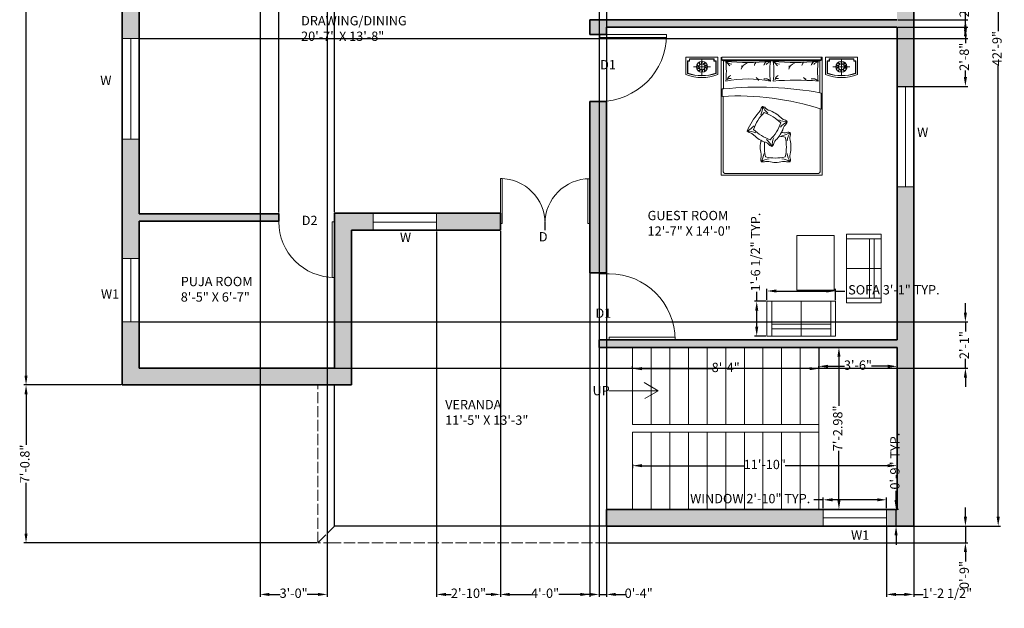
# Model space of a CAD drawing. Units: inches. Extents: x -34 to 523, y -544 to 92.
# Tile 1 of 2: x -11 to 518, y -544 to -227. Entities that reach past the tile are written whole.
import ezdxf

# ---------------------------------------------------------------- set-up
doc = ezdxf.new("R2010")
doc.units = ezdxf.units.IN
doc.linetypes.add('ACAD_ISO02W100', pattern=[15, 12, -3])
for name, color, linetype, lineweight in [('A-ANNO-DIMS', 2, 'Continuous', 18), ('A-ANNO-SYMB', 7, 'Continuous', 18), ('A-ANNO-TEXT', 7, 'Continuous', 18), ('A-AREA-IDEN', 7, 'Continuous', 25), ('A-DOOR', 4, 'Continuous', 18), ('A-FLOR', 7, 'Continuous', 25), ('A-FLOR-OVHD', 8, 'ACAD_ISO02W100', 18), ('A-FLOR-STRS', 7, 'Continuous', 18), ('A-GLAZ', 4, 'Continuous', 18), ('A-WALL', 7, 'Continuous', 35), ('furn', 28, 'Continuous', 18)]:
    doc.layers.add(name, color=color, linetype=linetype, lineweight=lineweight)
doc.layers.add('A-WALL-PATT', color=244, linetype='Continuous', lineweight=13, true_color=0x991b1e)
doc.styles.get("Standard").update_dxf_attribs({"font": 'arial.ttf'})
doc.dimstyles.new('ISO-25', dxfattribs={"dimtxt": 5, "dimasz": 5, "dimexe": 1.25, "dimexo": 0.625, "dimtad": 0, "dimlunit": 3, "dimtxsty": 'Standard', "dimcen": 2.5, "dimadec": 0, "dimazin": 0, "dimtfac": 1, "dimtmove": 0, "dimatfit": 3, "dimfxl": 1, "dimarcsym": 0})

# ---------------------------------------------------------------- blocks, each defined once
blk = doc.blocks.new('*U2')
for p, q in [((0, 0), (0, -6)), ((40, 0), (40, -6))]:
    blk.add_line(p, q)
blk.add_lwpolyline([(0, 0), (0, 40), (1.75, 40), (1.75, 0)], close=True)
blk.add_arc((0, 0), 40, 0, 90)
blk = doc.blocks.new('sofa-23')
at = {"color": 0, "linetype": 'ByBlock'}
for p, q in [((0, 0.74), (1.46, 0.74)), ((0, 0), (0, 0.74)), ((0.1, 0), (0.1, 0.74)), ((0.73, 0.74), (0.73, 0)), ((1.36, 0.74), (1.36, 0)), ((1.46, 0.74), (1.46, 0)), ((1.36, 0.25), (0.1, 0.25)), ((1.46, 0), (0, 0)), ((1.36, 0.15), (0.1, 0.15))]:
    blk.add_line(p, q, dxfattribs=at)
blk = doc.blocks.new('*D7')
at = {"layer": 'A-ANNO-DIMS', "color": 0, "lineweight": -2, "transparency": 16777216}
for p, q in [((418.12, -404.01), (418.12, -414.81)), ((460.12, -404.01), (460.12, -414.81)), ((423.12, -413.56), (431.86, -413.56)), ((455.12, -413.56), (446.39, -413.56))]:
    blk.add_line(p, q, dxfattribs=at)
at = {"layer": 'A-ANNO-DIMS', "color": 0, "transparency": 16777216}
for points in [[(423.12, -412.72), (423.12, -414.39), (418.12, -413.56)], [(455.12, -412.72), (455.12, -414.39), (460.12, -413.56)]]:
    blk.add_solid(points, dxfattribs=at)
at = {"layer": 'Defpoints', "color": 0, "transparency": 16777216}
for p in [(418.12, -403.38), (460.12, -403.38), (460.12, -413.56)]:
    blk.add_point(p, dxfattribs=at)
at = {"layer": 'A-ANNO-DIMS', "color": 0, "transparency": 16777216, "insert": (439.12, -413.56), "char_height": 5, "attachment_point": 5}
blk.add_mtext('3\'-6"', dxfattribs=at)
blk = doc.blocks.new('*D8')
at = {"layer": 'A-ANNO-DIMS', "color": 0, "lineweight": -2, "transparency": 16777216}
for p, q in [((318.12, -414.18), (318.12, -413.56)), ((323.12, -414.81), (360.85, -414.81)), ((413.12, -414.81), (375.4, -414.81)), ((418.12, -414.18), (418.12, -413.56))]:
    blk.add_line(p, q, dxfattribs=at)
at = {"layer": 'A-ANNO-DIMS', "color": 0, "transparency": 16777216}
for points in [[(323.12, -413.97), (323.12, -415.64), (318.12, -414.81)], [(413.12, -413.97), (413.12, -415.64), (418.12, -414.81)]]:
    blk.add_solid(points, dxfattribs=at)
at = {"layer": 'Defpoints', "color": 0, "transparency": 16777216}
for p in [(318.12, -414.81), (318.12, -414.81), (418.12, -414.81)]:
    blk.add_point(p, dxfattribs=at)
at = {"layer": 'A-ANNO-DIMS', "color": 0, "transparency": 16777216, "insert": (368.12, -414.81), "char_height": 5, "attachment_point": 5}
blk.add_mtext('8\'-4"', dxfattribs=at)
blk = doc.blocks.new('*D9')
at = {"layer": 'A-ANNO-DIMS', "color": 0, "lineweight": -2, "transparency": 16777216}
for p, q in [((418.75, -403.38), (430.17, -403.38)), ((428.92, -408.38), (428.92, -434.76)), ((428.92, -485.36), (428.92, -458.98)), ((418.75, -490.36), (430.17, -490.36))]:
    blk.add_line(p, q, dxfattribs=at)
at = {"layer": 'A-ANNO-DIMS', "color": 0, "transparency": 16777216}
for points in [[(428.09, -408.38), (429.75, -408.38), (428.92, -403.38)], [(428.09, -485.36), (429.75, -485.36), (428.92, -490.36)]]:
    blk.add_solid(points, dxfattribs=at)
at = {"layer": 'Defpoints', "color": 0, "transparency": 16777216}
for p in [(418.12, -403.38), (418.12, -490.36), (428.92, -490.36)]:
    blk.add_point(p, dxfattribs=at)
at = {"layer": 'A-ANNO-DIMS', "color": 0, "transparency": 16777216, "insert": (428.92, -446.87), "char_height": 5, "attachment_point": 5, "rotation": 90}
blk.add_mtext('7\'-2.98"', dxfattribs=at)
blk = doc.blocks.new('*D10')
at = {"layer": 'A-ANNO-DIMS', "color": 0, "lineweight": -2, "transparency": 16777216}
for p, q in [((318.12, -466.13), (318.12, -468.18)), ((323.12, -466.93), (378.2, -466.93)), ((455.12, -466.93), (400.04, -466.93)), ((460.12, -466.13), (460.12, -468.18))]:
    blk.add_line(p, q, dxfattribs=at)
at = {"layer": 'A-ANNO-DIMS', "color": 0, "transparency": 16777216}
for points in [[(323.12, -466.09), (323.12, -467.76), (318.12, -466.93)], [(455.12, -466.09), (455.12, -467.76), (460.12, -466.93)]]:
    blk.add_solid(points, dxfattribs=at)
at = {"layer": 'Defpoints', "color": 0, "transparency": 16777216}
for p in [(318.12, -465.51), (460.12, -465.51), (460.12, -466.93)]:
    blk.add_point(p, dxfattribs=at)
at = {"layer": 'A-ANNO-DIMS', "color": 0, "transparency": 16777216, "insert": (389.12, -466.93), "char_height": 5, "attachment_point": 5}
blk.add_mtext('11\'-10"', dxfattribs=at)
blk = doc.blocks.new('*D11')
at = {"layer": 'A-ANNO-DIMS', "color": 0, "lineweight": -2, "transparency": 16777216}
for p, q in [((43.5, -423.58), (-8.81, -423.58)), ((-7.56, -428.58), (-7.56, -455.82)), ((-7.56, -503.38), (-7.56, -476.14)), ((148.5, -508.38), (-8.81, -508.38))]:
    blk.add_line(p, q, dxfattribs=at)
at = {"layer": 'A-ANNO-DIMS', "color": 0, "transparency": 16777216}
for points in [[(-8.39, -428.58), (-6.73, -428.58), (-7.56, -423.58)], [(-8.39, -503.38), (-6.73, -503.38), (-7.56, -508.38)]]:
    blk.add_solid(points, dxfattribs=at)
at = {"layer": 'Defpoints', "color": 0, "transparency": 16777216}
for p in [(44.12, -423.58), (-7.56, -508.38), (149.12, -508.38)]:
    blk.add_point(p, dxfattribs=at)
at = {"layer": 'A-ANNO-DIMS', "color": 0, "transparency": 16777216, "insert": (-7.56, -465.98), "char_height": 5, "attachment_point": 5, "rotation": 90}
blk.add_mtext('7\'-0.8"', dxfattribs=at)
blk = doc.blocks.new('*D12')
at = {"layer": 'A-ANNO-DIMS', "color": 0, "lineweight": -2, "transparency": 16777216}
for p, q in [((0.5, 13.62), (-8.81, 13.62)), ((-7.56, 8.62), (-7.56, -192.86)), ((-7.56, -418.58), (-7.56, -217.1)), ((43.5, -423.58), (-8.81, -423.58))]:
    blk.add_line(p, q, dxfattribs=at)
at = {"layer": 'A-ANNO-DIMS', "color": 0, "transparency": 16777216}
for points in [[(-8.39, 8.62), (-6.73, 8.62), (-7.56, 13.62)], [(-8.39, -418.58), (-6.73, -418.58), (-7.56, -423.58)]]:
    blk.add_solid(points, dxfattribs=at)
at = {"layer": 'Defpoints', "color": 0, "transparency": 16777216}
for p in [(1.12, 13.62), (-7.56, -423.58), (44.12, -423.58)]:
    blk.add_point(p, dxfattribs=at)
at = {"layer": 'A-ANNO-DIMS', "color": 0, "transparency": 16777216, "insert": (-7.56, -204.98), "char_height": 5, "attachment_point": 5, "rotation": 90}
blk.add_mtext('36\'-5.2"', dxfattribs=at)
blk = doc.blocks.new('*D14')
at = {"layer": 'A-ANNO-DIMS', "color": 0, "lineweight": -2, "transparency": 16777216}
for p, q in [((469.75, 13.62), (515.68, 13.62)), ((514.43, 8.62), (514.43, -233.57)), ((514.43, -494.38), (514.43, -252.2)), ((469.75, -499.38), (515.68, -499.38))]:
    blk.add_line(p, q, dxfattribs=at)
at = {"layer": 'A-ANNO-DIMS', "color": 0, "transparency": 16777216}
for points in [[(513.6, 8.62), (515.26, 8.62), (514.43, 13.62)], [(513.6, -494.38), (515.26, -494.38), (514.43, -499.38)]]:
    blk.add_solid(points, dxfattribs=at)
at = {"layer": 'Defpoints', "color": 0, "transparency": 16777216}
for p in [(469.12, 13.62), (469.12, -499.38), (514.43, -499.38)]:
    blk.add_point(p, dxfattribs=at)
at = {"layer": 'A-ANNO-DIMS', "color": 0, "transparency": 16777216, "insert": (514.43, -242.88), "char_height": 5, "attachment_point": 5, "rotation": 90}
blk.add_mtext('42\'-9"', dxfattribs=at)
blk = doc.blocks.new('BED-DOUBLE')
for p, q in [((0.94, 61.53), (53.14, 61.53)), ((1.21, 61.99), (1.21, 46.38)), ((52.84, 61.99), (52.84, 44.35))]:
    blk.add_line(p, q)
for points in [[(0, 63.46), (0, 0), (54.08, 0), (54.08, 63.46)], [(53.58, 63.46), (53.58, 61.99), (0.31, 61.99), (0.31, 63.46), (54.08, 63.46)]]:
    blk.add_lwpolyline(points)
for points in [[(2.4, 50.65, 0.058596), (2.4, 61.1, 0.036889), (26.34, 61.1, 0.052163), (26.34, 50.65, 0.093111)], [(27.89, 50.65, 0.058596), (27.89, 61.1, 0.036648), (51.99, 61.1, 0.052163), (51.99, 50.65, 0.036967)], [(0.47, 46.38), (1.21, 46.38, -0.072944), (53.58, 44.2), (53.58, 35.53, 0.092568), (0.47, 42.4)]]:
    blk.add_lwpolyline(points, format="xyb", close=True)
for points in [[(0.94, 42.43), (0.94, 2.5, 0.414214), (2.5, 0.94), (51.58, 0.94, 0.414214), (53.14, 2.5), (53.14, 35.68)], [(21.24, 32.47, 0.091296), (22.19, 37.05, 0.091296), (25.07, 33.37, 0.091296)], [(17.36, 24.65, 0.111006), (26.29, 19.1, 0.119549), (31.92, 28.13, 0.107813), (23.02, 33.71)], [(22.97, 33.69, 0.121865), (17.36, 24.65, 0.121865)], [(18.5, 22.82, 0.091296), (13.92, 23.79, 0.091296), (17.61, 26.66, 0.091296)], [(27.19, 15.52, 0.159461), (28.4, 17.67, -0.076283), (29.36, 19, 0.115075), (33.28, 25.3, -0.076283), (34.06, 26.75, 0.159461), (35.45, 28.79)], [(30.88, 29.75, 0.091296), (35.45, 28.79, 0.091296), (31.76, 25.91, 0.091296)], [(32.56, 21.35, 0.091296), (36.96, 22.96, 0.091296), (35.34, 18.57, 0.091296)], [(36.96, 7.33, 0.159461), (36.85, 9.79, -0.076283), (36.96, 11.43, 0.115075), (36.96, 18.85, -0.076283), (36.85, 20.49, 0.159461), (36.96, 22.96)], [(23.79, 9.88, 0.111006), (34.31, 9.89, 0.119549), (34.31, 20.53, 0.033212), (31.08, 21.02)], [(28.14, 20.1, 0.091296), (27.19, 15.52, 0.091296), (24.3, 19.2)], [(25.72, 8.93, 0.091296), (21.33, 7.33, 0.091296), (22.94, 11.71, 0.091296)], [(35.34, 11.71, 0.091296), (36.96, 7.33, 0.091296), (32.56, 8.93)]]:
    blk.add_lwpolyline(points, format="xyb")
for centre, radius, start, end in [((0.94, 62.47), 0.938, 180, 270), ((7.95, 69.83), 10.35, 237.5379, 257.5233), ((-5.44, 51.33), 12.52, 36.4935, 51.2792), ((8.37, 58.13), 2.6, 335.8927, 16.1192), ((15.89, 54.9), 5.79, 96.6849, 148.3182), ((21.75, 58.2), 4.06, 141.8174, 169.8987), ((26.89, 57.62), 4.37, 130.5354, 160.3558), ((29.62, 53.94), 7.88, 114.6457, 134.1585), ((20.06, 51.33), 12.52, 36.4935, 51.2792), ((33.45, 69.83), 10.35, 237.5379, 257.5233), ((33.87, 58.13), 2.6, 335.8927, 16.1192), ((41.39, 54.9), 5.79, 96.6849, 148.3182), ((47.25, 58.2), 4.06, 141.8174, 169.8987), ((52.39, 57.62), 4.37, 130.5354, 160.3558), ((55.11, 53.94), 7.88, 114.6457, 134.1585), ((53.14, 62.47), 0.938, 270, 0), ((6.51, 50.41), 3.47, 114.2916, 160.9896), ((32.01, 50.41), 3.47, 114.2916, 160.9896), ((4.71, 49.68), 2.38, 76.4823, 128.5563), ((9.44, 43.38), 13.05, 36.2085, 45.0849), ((19.1, 51.09), 0.876, 353.7543, 77.2187), ((23.28, 47.66), 4.27, 44.406, 96.8342), ((24.08, 49.15), 2.71, 33.6349, 90.8456), ((30.2, 49.68), 2.38, 76.4823, 128.5563), ((34.94, 43.38), 13.05, 36.2085, 45.0849), ((44.59, 51.09), 0.876, 353.7543, 77.2187), ((48.78, 47.66), 4.27, 44.406, 96.8342), ((49.58, 49.15), 2.71, 33.6349, 90.8456), ((24.86, 34.13), 3.96, 132.4658, 168.7065), ((21.14, 33.37), 3.82, 37.2937, 74.0973), ((45.61, 10.83), 34.23, 138.3818, 157.7644), ((16.14, 37.37), 5.43, 315.5854, 333.0343), ((27.43, 40.04), 5.43, 233.2983, 250.7472), ((20.42, 19.44), 16.33, 45.1307, 71.3884), ((35.73, 34.9), 5.43, 225.7718, 243.2208), ((32.63, 26.46), 3.66, 39.4726, 79.6505), ((16.84, 26.47), 3.96, 222.6522, 258.8929), ((13.63, 17.74), 5.43, 45.7718, 63.2208), ((28.94, 33.2), 16.33, 225.1307, 251.3884), ((29.14, 7.07), 16.33, 77.0576, 78.7033), ((33.96, 28.3), 5.43, 257.6988, 275.1477), ((35.79, 19.49), 3.66, 71.3996, 111.5774), ((37.23, 15.14), 16.33, 166.8711, 193.1289), ((45.29, 15.25), 22.16, 173.1956, 194.0284), ((21.93, 12.6), 5.43, 53.2983, 70.7472), ((28.71, 19.79), 4.53, 218.7754, 250.3571), ((16.03, 10.26), 5.43, 355.0387, 12.4877), ((25.14, 8.39), 3.96, 159.3666, 195.6073), ((22.38, 11.14), 3.96, 254.5791, 290.8198), ((24.28, 2.04), 5.43, 77.6988, 95.1477), ((29.09, 23.26), 16.33, 257.0576, 283.3153), ((34.04, 2.07), 5.43, 85.2252, 102.6741), ((35.99, 11.75), 4.53, 250.7023, 282.284)]:
    blk.add_arc(centre, radius, start, end)
blk = doc.blocks.new('NIGHTSTAND-L')
for p, q in [((4.18, 5.76), (13.19, 5.76)), ((8.69, 1.26), (8.69, 10.27))]:
    blk.add_line(p, q)
blk.add_lwpolyline([(0, 1.56), (0, 10.94), (17.19, 10.94), (17.19, 1.56, -0.181818)], format="xyb", close=True)
for points in [[(1.97, 10), (1.97, 8.97), (0.94, 8.97)], [(2.06, 10), (2.06, 8.88), (0.94, 8.88)], [(1.97, 10), (15.22, 10)], [(1.97, 9.91), (15.22, 9.91)], [(15.13, 10), (15.13, 8.88), (16.26, 8.88)], [(15.22, 10), (15.22, 8.97), (16.26, 8.97)]]:
    blk.add_lwpolyline(points)
for points in [[(16.26, 8.97), (16.26, 2.22, -0.167087), (0.94, 2.22), (0.94, 8.97)], [(16.16, 8.97), (16.16, 2.28, -0.165559), (1.03, 2.28), (1.03, 8.97)]]:
    blk.add_lwpolyline(points, format="xyb")
for radius in [2.94, 1.6]:
    blk.add_circle((8.69, 5.76), radius)
for centre, radius, start, end in [((6.65, 6.51), 1.44, 232.3002, 292.538), ((7.6, 7.7), 1.89, 208.17, 254.4897), ((7.47, 7.56), 1.44, 196.3002, 256.538), ((8.95, 7.97), 1.89, 172.17, 218.4897), ((8.76, 7.93), 1.44, 160.3002, 220.538), ((10.19, 7.4), 1.89, 136.17, 182.4897), ((10.02, 7.47), 1.44, 124.3002, 184.538), ((10.86, 6.2), 1.89, 100.17, 146.4897), ((10.77, 6.36), 1.44, 88.3002, 148.538), ((10.7, 4.83), 1.89, 64.17, 110.4897), ((10.72, 5.02), 1.44, 52.3002, 112.538), ((9.9, 3.97), 1.44, 16.3002, 76.538), ((9.77, 3.83), 1.89, 28.17, 74.4897), ((6.67, 6.69), 1.89, 244.17, 290.4897), ((6.6, 5.17), 1.44, 268.3002, 328.538), ((6.51, 5.33), 1.89, 280.17, 326.4897), ((7.35, 4.06), 1.44, 304.3002, 4.538), ((7.18, 4.13), 1.89, 316.17, 2.4897), ((8.61, 3.6), 1.44, 340.3002, 40.538), ((8.42, 3.56), 1.89, 352.17, 38.4897)]:
    blk.add_arc(centre, radius, start, end)
blk = doc.blocks.new('NIGHTSTAND-R')
for p, q in [((13.02, 5.76), (4, 5.76)), ((8.51, 1.25), (8.51, 10.27))]:
    blk.add_line(p, q)
blk.add_lwpolyline([(17.19, 1.56), (17.19, 10.94), (0, 10.94), (0, 1.56, 0.181818)], format="xyb", close=True)
for points in [[(1.97, 10), (1.97, 8.97), (0.94, 8.97)], [(2.06, 10), (2.06, 8.88), (0.94, 8.88)], [(15.22, 10), (1.97, 10)], [(15.22, 9.91), (1.97, 9.91)], [(15.13, 10), (15.13, 8.88), (16.26, 8.88)], [(15.22, 10), (15.22, 8.97), (16.26, 8.97)]]:
    blk.add_lwpolyline(points)
for points in [[(0.94, 8.97), (0.94, 2.22, 0.167087), (16.26, 2.22), (16.26, 8.97)], [(1.03, 8.97), (1.03, 2.28, 0.165559), (16.16, 2.28), (16.16, 8.97)]]:
    blk.add_lwpolyline(points, format="xyb")
for radius in [2.94, 1.6]:
    blk.add_circle((8.51, 5.76), radius)
for centre, radius, start, end in [((6.47, 5.02), 1.44, 67.462, 127.6998), ((6.49, 4.83), 1.89, 69.5103, 115.83), ((7.42, 3.82), 1.89, 105.5103, 151.83), ((7.3, 3.96), 1.44, 103.462, 163.6998), ((6.43, 6.36), 1.44, 31.462, 91.6998), ((6.33, 6.19), 1.89, 33.5103, 79.83), ((7.17, 7.47), 1.44, 355.462, 55.6998), ((7, 7.39), 1.89, 357.5103, 43.83), ((8.43, 7.92), 1.44, 319.462, 19.6998), ((8.46, 8.05), 1.89, 321.5103, 7.83), ((10.76, 6.58), 1.44, 247.462, 307.6998), ((9.93, 7.64), 1.44, 283.462, 343.6998), ((9.81, 7.78), 1.89, 285.5103, 331.83), ((8.77, 3.55), 1.89, 141.5103, 187.83), ((8.58, 3.6), 1.44, 139.462, 199.6998), ((10.02, 4.13), 1.89, 177.5103, 223.83), ((9.84, 4.05), 1.44, 175.462, 235.6998), ((10.69, 5.33), 1.89, 213.5103, 259.83), ((10.59, 5.16), 1.44, 211.462, 271.6998), ((10.74, 6.77), 1.89, 249.5103, 295.83)]:
    blk.add_arc(centre, radius, start, end)
blk = doc.blocks.new('WIN-34IN')
blk.add_line((4.5, 34), (4.5, 0))
blk.add_lwpolyline([(9, 34), (9, 0), (0, 0), (0, 34)], close=True)
blk = doc.blocks.new('WIN-54IN')
blk.add_line((4.5, 54), (4.5, 0))
blk.add_lwpolyline([(0, 54), (9, 54), (9, 0), (0, 0)], close=True)
blk = doc.blocks.new('*D20')
at = {"layer": 'A-ANNO-DIMS', "color": 0, "lineweight": -2, "transparency": 16777216}
for p, q in [((420.49, -485.26), (415.49, -485.26)), ((420.49, -489.73), (420.49, -484.01)), ((449.49, -485.26), (425.49, -485.26)), ((454.49, -489.73), (454.49, -484.01))]:
    blk.add_line(p, q, dxfattribs=at)
at = {"layer": 'A-ANNO-DIMS', "color": 0, "transparency": 16777216}
for points in [[(425.49, -484.42), (425.49, -486.09), (420.49, -485.26)], [(449.49, -484.42), (449.49, -486.09), (454.49, -485.26)]]:
    blk.add_solid(points, dxfattribs=at)
at = {"layer": 'Defpoints', "color": 0, "transparency": 16777216}
for p in [(420.49, -485.26), (420.49, -490.36), (454.49, -490.36)]:
    blk.add_point(p, dxfattribs=at)
at = {"layer": 'A-ANNO-DIMS', "color": 0, "transparency": 16777216, "insert": (381.28, -485.26), "char_height": 5, "attachment_point": 5}
blk.add_mtext('WINDOW 2\'-10" TYP.', dxfattribs=at)
blk = doc.blocks.new('*D21')
at = {"layer": 'A-ANNO-DIMS', "color": 0, "lineweight": -2, "transparency": 16777216}
for p, q in [((459.59, -485.36), (459.59, -480.36)), ((455.11, -490.36), (460.84, -490.36)), ((459.59, -499.36), (459.59, -490.36)), ((455.11, -499.36), (460.84, -499.36)), ((459.59, -504.36), (459.59, -509.36))]:
    blk.add_line(p, q, dxfattribs=at)
at = {"layer": 'A-ANNO-DIMS', "color": 0, "transparency": 16777216}
for points in [[(458.75, -485.36), (460.42, -485.36), (459.59, -490.36)], [(458.75, -504.36), (460.42, -504.36), (459.59, -499.36)]]:
    blk.add_solid(points, dxfattribs=at)
at = {"layer": 'Defpoints', "color": 0, "transparency": 16777216}
for p in [(454.49, -490.36), (459.59, -490.36), (454.49, -499.36)]:
    blk.add_point(p, dxfattribs=at)
at = {"layer": 'A-ANNO-DIMS', "color": 0, "transparency": 16777216, "insert": (459.59, -464.49), "char_height": 5, "attachment_point": 5, "rotation": 90}
blk.add_mtext('0\'-9" TYP.', dxfattribs=at)
blk = doc.blocks.new('*D30')
at = {"layer": 'A-ANNO-DIMS', "color": 0, "lineweight": -2, "transparency": 16777216}
for p, q in [((390.29, -378.01), (390.29, -371.86)), ((395.29, -373.11), (422.1, -373.11)), ((427.1, -378.01), (427.1, -371.86)), ((427.1, -373.11), (432.1, -373.11))]:
    blk.add_line(p, q, dxfattribs=at)
at = {"layer": 'A-ANNO-DIMS', "color": 0, "transparency": 16777216}
for points in [[(395.29, -372.28), (395.29, -373.95), (390.29, -373.11)], [(422.1, -372.28), (422.1, -373.95), (427.1, -373.11)]]:
    blk.add_solid(points, dxfattribs=at)
at = {"layer": 'Defpoints', "color": 0, "transparency": 16777216}
for p in [(427.1, -373.11), (390.29, -378.64), (427.1, -378.64)]:
    blk.add_point(p, dxfattribs=at)
at = {"layer": 'A-ANNO-DIMS', "color": 0, "transparency": 16777216, "insert": (458.43, -373.11), "char_height": 5, "attachment_point": 5}
blk.add_mtext('SOFA 3\'-1" TYP.', dxfattribs=at)
blk = doc.blocks.new('*D31')
at = {"layer": 'A-ANNO-DIMS', "color": 0, "lineweight": -2, "transparency": 16777216}
for p, q in [((384.77, -378.64), (384.77, -373.64)), ((389.66, -378.64), (383.52, -378.64)), ((384.77, -392.29), (384.77, -383.64)), ((389.66, -397.29), (383.52, -397.29))]:
    blk.add_line(p, q, dxfattribs=at)
at = {"layer": 'A-ANNO-DIMS', "color": 0, "transparency": 16777216}
for points in [[(383.93, -383.64), (385.6, -383.64), (384.77, -378.64)], [(383.93, -392.29), (385.6, -392.29), (384.77, -397.29)]]:
    blk.add_solid(points, dxfattribs=at)
at = {"layer": 'Defpoints', "color": 0, "transparency": 16777216}
for p in [(384.77, -378.64), (390.29, -378.64), (390.29, -397.29)]:
    blk.add_point(p, dxfattribs=at)
at = {"layer": 'A-ANNO-DIMS', "color": 0, "transparency": 16777216, "insert": (384.77, -352.18), "char_height": 5, "attachment_point": 5, "rotation": 90}
blk.add_mtext('1\'-6 1/2" TYP.', dxfattribs=at)
blk = doc.blocks.new('*D32')
at = {"layer": 'A-ANNO-DIMS', "color": 0, "lineweight": -2, "transparency": 16777216}
for p, q in [((118.12, -168.01), (118.12, -537.33)), ((154.12, -168.01), (154.12, -537.33)), ((123.12, -536.08), (128.86, -536.08)), ((149.12, -536.08), (143.39, -536.08))]:
    blk.add_line(p, q, dxfattribs=at)
at = {"layer": 'A-ANNO-DIMS', "color": 0, "transparency": 16777216}
for points in [[(123.12, -535.25), (123.12, -536.92), (118.12, -536.08)], [(149.12, -535.25), (149.12, -536.92), (154.12, -536.08)]]:
    blk.add_solid(points, dxfattribs=at)
at = {"layer": 'Defpoints', "color": 0, "transparency": 16777216}
for p in [(118.12, -167.38), (154.12, -167.38), (154.12, -536.08)]:
    blk.add_point(p, dxfattribs=at)
at = {"layer": 'A-ANNO-DIMS', "color": 0, "transparency": 16777216, "insert": (136.12, -536.08), "char_height": 5, "attachment_point": 5}
blk.add_mtext('3\'-0"', dxfattribs=at)
blk = doc.blocks.new('*D33')
at = {"layer": 'A-ANNO-DIMS', "color": 0, "lineweight": -2, "transparency": 16777216}
for p, q in [((128.12, -330.95), (128.12, 42.7)), ((158.12, -330.76), (158.12, 42.7)), ((133.12, 41.45), (135.81, 41.45)), ((153.12, 41.45), (150.44, 41.45))]:
    blk.add_line(p, q, dxfattribs=at)
at = {"layer": 'A-ANNO-DIMS', "color": 0, "transparency": 16777216}
for points in [[(133.12, 42.29), (133.12, 40.62), (128.12, 41.45)], [(153.12, 42.29), (153.12, 40.62), (158.12, 41.45)]]:
    blk.add_solid(points, dxfattribs=at)
at = {"layer": 'Defpoints', "color": 0, "transparency": 16777216}
for p in [(158.12, 41.45), (128.12, -331.58), (158.12, -331.38)]:
    blk.add_point(p, dxfattribs=at)
at = {"layer": 'A-ANNO-DIMS', "color": 0, "transparency": 16777216, "insert": (143.12, 41.45), "char_height": 5, "attachment_point": 5}
blk.add_mtext('2\'-6"', dxfattribs=at)
blk = doc.blocks.new('*D34')
at = {"layer": 'A-ANNO-DIMS', "color": 0, "lineweight": -2, "transparency": 16777216}
for p, q in [((247.12, -341.01), (247.12, -537.33)), ((295.12, -341.08), (295.12, -537.33)), ((252.12, -536.08), (263.75, -536.08)), ((290.12, -536.08), (278.5, -536.08))]:
    blk.add_line(p, q, dxfattribs=at)
at = {"layer": 'A-ANNO-DIMS', "color": 0, "transparency": 16777216}
for points in [[(252.12, -535.25), (252.12, -536.92), (247.12, -536.08)], [(290.12, -535.25), (290.12, -536.92), (295.12, -536.08)]]:
    blk.add_solid(points, dxfattribs=at)
at = {"layer": 'Defpoints', "color": 0, "transparency": 16777216}
for p in [(247.12, -340.38), (295.12, -340.45), (295.12, -536.08)]:
    blk.add_point(p, dxfattribs=at)
at = {"layer": 'A-ANNO-DIMS', "color": 0, "transparency": 16777216, "insert": (271.12, -536.08), "char_height": 5, "attachment_point": 5}
blk.add_mtext('4\'-0"', dxfattribs=at)
blk = doc.blocks.new('*D37')
at = {"layer": 'A-ANNO-DIMS', "color": 0, "lineweight": -2, "transparency": 16777216}
for p, q in [((300.12, -168.01), (300.12, -537.33)), ((304.12, -164.01), (304.12, -537.33)), ((295.12, -536.08), (290.12, -536.08)), ((300.12, -536.08), (304.12, -536.08)), ((309.12, -536.08), (314.12, -536.08))]:
    blk.add_line(p, q, dxfattribs=at)
at = {"layer": 'A-ANNO-DIMS', "color": 0, "transparency": 16777216}
for points in [[(295.12, -535.25), (295.12, -536.92), (300.12, -536.08)], [(309.12, -535.25), (309.12, -536.92), (304.12, -536.08)]]:
    blk.add_solid(points, dxfattribs=at)
at = {"layer": 'Defpoints', "color": 0, "transparency": 16777216}
for p in [(304.12, -163.38), (300.12, -167.38), (304.12, -536.08)]:
    blk.add_point(p, dxfattribs=at)
at = {"layer": 'A-ANNO-DIMS', "color": 0, "transparency": 16777216, "insert": (321.4, -536.08), "char_height": 5, "attachment_point": 5}
blk.add_mtext('0\'-4"', dxfattribs=at)
blk = doc.blocks.new('*D41')
at = {"layer": 'A-ANNO-DIMS', "color": 0, "lineweight": -2, "transparency": 16777216}
for p, q in [((53.75, -167.38), (498.07, -167.38)), ((496.82, -172.38), (496.82, -193.25)), ((496.82, -232.53), (496.82, -211.67)), ((53.78, -237.53), (498.07, -237.53))]:
    blk.add_line(p, q, dxfattribs=at)
at = {"layer": 'A-ANNO-DIMS', "color": 0, "transparency": 16777216}
for points in [[(495.99, -172.38), (497.66, -172.38), (496.82, -167.38)], [(495.99, -232.53), (497.66, -232.53), (496.82, -237.53)]]:
    blk.add_solid(points, dxfattribs=at)
at = {"layer": 'Defpoints', "color": 0, "transparency": 16777216}
for p in [(53.12, -167.38), (53.16, -237.53), (496.82, -237.53)]:
    blk.add_point(p, dxfattribs=at)
at = {"layer": 'A-ANNO-DIMS', "color": 0, "transparency": 16777216, "insert": (496.82, -202.46), "char_height": 5, "attachment_point": 5, "rotation": 90}
blk.add_mtext('5\'-10"', dxfattribs=at)
blk = doc.blocks.new('*D42')
at = {"layer": 'A-ANNO-DIMS', "color": 0, "lineweight": -2, "transparency": 16777216}
for p, q in [((496.82, -384.72), (496.82, -379.72)), ((53.75, -389.72), (498.07, -389.72)), ((496.82, -389.72), (496.82, -394.84)), ((496.82, -414.58), (496.82, -409.46)), ((53.75, -414.58), (498.07, -414.58)), ((496.82, -419.58), (496.82, -424.58))]:
    blk.add_line(p, q, dxfattribs=at)
at = {"layer": 'A-ANNO-DIMS', "color": 0, "transparency": 16777216}
for points in [[(495.99, -384.72), (497.66, -384.72), (496.82, -389.72)], [(495.99, -419.58), (497.66, -419.58), (496.82, -414.58)]]:
    blk.add_solid(points, dxfattribs=at)
at = {"layer": 'Defpoints', "color": 0, "transparency": 16777216}
for p in [(53.12, -389.72), (53.12, -414.58), (496.82, -414.58)]:
    blk.add_point(p, dxfattribs=at)
at = {"layer": 'A-ANNO-DIMS', "color": 0, "transparency": 16777216, "insert": (496.82, -402.15), "char_height": 5, "attachment_point": 5, "rotation": 90}
blk.add_mtext('2\'-1"', dxfattribs=at)
blk = doc.blocks.new('*D44')
at = {"layer": 'A-ANNO-DIMS', "color": 0, "lineweight": -2, "transparency": 16777216}
for p, q in [((460.75, -231.38), (498.07, -231.38)), ((496.82, -236.38), (496.82, -239.98)), ((496.82, -258.2), (496.82, -254.61)), ((460.75, -263.2), (498.07, -263.2))]:
    blk.add_line(p, q, dxfattribs=at)
at = {"layer": 'A-ANNO-DIMS', "color": 0, "transparency": 16777216}
for points in [[(495.99, -236.38), (497.66, -236.38), (496.82, -231.38)], [(495.99, -258.2), (497.66, -258.2), (496.82, -263.2)]]:
    blk.add_solid(points, dxfattribs=at)
at = {"layer": 'Defpoints', "color": 0, "transparency": 16777216}
for p in [(460.12, -231.38), (460.12, -263.2), (496.82, -263.2)]:
    blk.add_point(p, dxfattribs=at)
at = {"layer": 'A-ANNO-DIMS', "color": 0, "transparency": 16777216, "insert": (496.82, -247.29), "char_height": 5, "attachment_point": 5, "rotation": 90}
blk.add_mtext('2\'-8"', dxfattribs=at)
blk = doc.blocks.new('*D45')
at = {"layer": 'A-ANNO-DIMS', "color": 0, "lineweight": -2, "transparency": 16777216}
for p, q in [((212.88, -341.18), (212.88, -537.33)), ((247.12, -341.01), (247.12, -537.33)), ((217.88, -536.08), (220.75, -536.08)), ((242.12, -536.08), (239.26, -536.08))]:
    blk.add_line(p, q, dxfattribs=at)
at = {"layer": 'A-ANNO-DIMS', "color": 0, "transparency": 16777216}
for points in [[(217.88, -535.25), (217.88, -536.92), (212.88, -536.08)], [(242.12, -535.25), (242.12, -536.92), (247.12, -536.08)]]:
    blk.add_solid(points, dxfattribs=at)
at = {"layer": 'Defpoints', "color": 0, "transparency": 16777216}
for p in [(212.88, -340.56), (247.12, -340.38), (247.12, -536.08)]:
    blk.add_point(p, dxfattribs=at)
at = {"layer": 'A-ANNO-DIMS', "color": 0, "transparency": 16777216, "insert": (230, -536.08), "char_height": 5, "attachment_point": 5}
blk.add_mtext('2\'-10"', dxfattribs=at)
blk = doc.blocks.new('*D46')
at = {"layer": 'A-ANNO-DIMS', "color": 0, "lineweight": -2, "transparency": 16777216}
for p, q in [((454.49, -499.98), (454.49, -537.33)), ((469.12, -500.01), (469.12, -537.33)), ((459.49, -536.08), (464.12, -536.08)), ((469.12, -536.08), (474.12, -536.08))]:
    blk.add_line(p, q, dxfattribs=at)
at = {"layer": 'A-ANNO-DIMS', "color": 0, "transparency": 16777216}
for points in [[(459.49, -535.25), (459.49, -536.92), (454.49, -536.08)], [(464.12, -535.25), (464.12, -536.92), (469.12, -536.08)]]:
    blk.add_solid(points, dxfattribs=at)
at = {"layer": 'Defpoints', "color": 0, "transparency": 16777216}
for p in [(454.49, -499.36), (469.12, -499.38), (469.12, -536.08)]:
    blk.add_point(p, dxfattribs=at)
at = {"layer": 'A-ANNO-DIMS', "color": 0, "transparency": 16777216, "insert": (486.99, -536.08), "char_height": 5, "attachment_point": 5}
blk.add_mtext('1\'-2 1/2"', dxfattribs=at)
blk = doc.blocks.new('*D47')
at = {"layer": 'A-ANNO-DIMS', "color": 0, "lineweight": -2, "transparency": 16777216}
for p, q in [((496.82, -494.38), (496.82, -489.38)), ((304.75, -499.38), (498.07, -499.38)), ((496.82, -499.38), (496.82, -508.38)), ((304.75, -508.38), (498.07, -508.38)), ((496.82, -513.38), (496.82, -518.38))]:
    blk.add_line(p, q, dxfattribs=at)
at = {"layer": 'A-ANNO-DIMS', "color": 0, "transparency": 16777216}
for points in [[(495.99, -494.38), (497.66, -494.38), (496.82, -499.38)], [(495.99, -513.38), (497.66, -513.38), (496.82, -508.38)]]:
    blk.add_solid(points, dxfattribs=at)
at = {"layer": 'Defpoints', "color": 0, "transparency": 16777216}
for p in [(304.12, -499.38), (304.12, -508.38), (496.82, -508.38)]:
    blk.add_point(p, dxfattribs=at)
at = {"layer": 'A-ANNO-DIMS', "color": 0, "transparency": 16777216, "insert": (496.82, -525.65), "char_height": 5, "attachment_point": 5, "rotation": 90}
blk.add_mtext('0\'-9"', dxfattribs=at)
blk = doc.blocks.new('*D48')
at = {"layer": 'A-ANNO-DIMS', "color": 0, "lineweight": -2, "transparency": 16777216}
for p, q in [((496.82, -193.05), (496.82, -188.05)), ((460.75, -198.05), (498.07, -198.05)), ((496.82, -198.05), (496.82, -199.58)), ((496.82, -227.38), (496.82, -225.86)), ((460.75, -227.38), (498.07, -227.38)), ((496.82, -232.38), (496.82, -237.38))]:
    blk.add_line(p, q, dxfattribs=at)
at = {"layer": 'A-ANNO-DIMS', "color": 0, "transparency": 16777216}
for points in [[(495.99, -193.05), (497.66, -193.05), (496.82, -198.05)], [(495.99, -232.38), (497.66, -232.38), (496.82, -227.38)]]:
    blk.add_solid(points, dxfattribs=at)
at = {"layer": 'Defpoints', "color": 0, "transparency": 16777216}
for p in [(460.12, -198.05), (460.12, -227.38), (496.82, -227.38)]:
    blk.add_point(p, dxfattribs=at)
at = {"layer": 'A-ANNO-DIMS', "color": 0, "transparency": 16777216, "insert": (496.82, -212.72), "char_height": 5, "attachment_point": 5, "rotation": 90}
blk.add_mtext('2\'-5 1/2"', dxfattribs=at)

msp = doc.modelspace()

# ---------------------------------------------------------------- hatches: boundary and pattern name
at = {"layer": 'A-WALL-PATT'}
h = msp.add_hatch(color=256, dxfattribs=at)
h.dxf.hatch_style = 1
h.paths.add_polyline_path([(10.124, -43.915), (124.749, -43.915), (124.749, -34.915), (1.124, -34.915), (1.124, -83.244), (10.124, -83.244)])
h.paths.add_polyline_path([(10.124, -117.244), (1.124, -117.244), (1.124, -172.382), (10.124, -172.382), (44.124, -172.382), (44.124, -237.534), (53.124, -237.534), (53.124, -172.382), (53.124, -167.382), (118.124, -167.382), (118.124, -163.382), (10.124, -163.382)])
h.paths.add_polyline_path([(264.093, -163.382), (158.124, -163.382), (158.124, 4.618), (224.085, 4.618), (224.085, 13.618), (158.124, 13.618), (154.124, 13.618), (154.124, -34.915), (154.124, -39.302), (154.124, -68.549), (154.124, -167.382), (264.093, -167.382)])
h.paths.add_polyline_path([(304.124, 4.618), (355.273, 4.618), (355.273, 13.618), (258.085, 13.618), (258.085, 4.618), (300.124, 4.618), (300.124, -167.382), (304.124, -167.382), (315.124, -167.382), (315.124, -163.382), (304.124, -163.382)])
h.paths.add_polyline_path([(469.124, 13.618), (389.273, 13.618), (389.273, 4.618), (460.124, 4.618), (460.124, -67.595), (469.124, -67.595)])
h.paths.add_polyline_path([(469.124, -121.595), (460.124, -121.595), (460.124, -163.382), (351.124, -163.382), (351.124, -167.382), (351.124, -197.382), (355.124, -197.382), (355.124, -167.382), (460.124, -167.382), (460.124, -180.053), (469.124, -180.053)])
h.paths.add_polyline_path([(469.124, -198.053), (460.124, -198.053), (460.124, -227.382), (295.124, -227.382), (295.124, -231.382), (295.124, -235.382), (300.506, -235.382), (304.124, -235.382), (304.124, -231.382), (460.124, -231.382), (460.124, -263.203), (469.124, -263.203)])
h.paths.add_polyline_path([(469.124, -317.203), (460.124, -317.203), (460.124, -399.382), (300.124, -399.382), (300.124, -403.382), (460.124, -403.382), (460.124, -490.382), (454.486, -490.382), (454.486, -499.382), (469.124, -499.382)])
h = msp.add_hatch(color=256, dxfattribs=at)
h.dxf.hatch_style = 1
h.paths.add_polyline_path([(167.124, -340.382), (178.882, -340.382), (178.882, -331.382), (167.124, -331.382), (158.124, -331.382), (158.124, -335.878), (158.124, -365.853), (158.124, -414.58), (53.124, -414.58), (53.124, -389.717), (44.124, -389.717), (44.124, -423.58), (53.124, -423.58), (158.124, -423.58), (167.124, -423.58)])
h.paths.add_polyline_path([(53.124, -291.534), (44.124, -291.534), (44.124, -355.717), (53.124, -355.717), (53.124, -335.58), (128.124, -335.58), (128.124, -331.58), (53.124, -331.58)])
h.paths.add_polyline_path([(247.124, -331.382), (212.882, -331.382), (212.882, -340.382), (247.124, -340.382)])
h.paths.add_polyline_path([(304.124, -271.382), (295.124, -271.382), (295.124, -363.382), (300.124, -363.382), (304.124, -363.382)])
h.paths.add_polyline_path([(420.486, -490.382), (304.124, -490.382), (304.124, -499.382), (420.486, -499.382)])

# ---------------------------------------------------------------- linework, layer by layer
at = {"layer": 'A-ANNO-SYMB'}
for p, q in [((331.866, -426.686), (324.336, -422.339)), ((305.318, -426.686), (331.866, -426.686)), ((331.866, -426.686), (324.633, -430.862))]:
    msp.add_line(p, q, dxfattribs=at)
at = {"layer": 'A-FLOR'}
for p, q in [((158.124, -499.382), (158.124, -423.58)), ((304.124, -499.382), (158.124, -499.382))]:
    msp.add_line(p, q, dxfattribs=at)
at = {"layer": 'A-FLOR-OVHD', "ltscale": 0.5}
for p, q in [((149.124, -508.382), (149.124, -423.58)), ((149.124, -508.382), (158.124, -499.382)), ((304.124, -499.382), (304.124, -508.382)), ((158.124, -508.382), (149.124, -508.382)), ((304.124, -508.382), (158.124, -508.382))]:
    msp.add_line(p, q, dxfattribs=at)
at = {"layer": 'A-FLOR-STRS'}
for p, q in [((318.124, -403.382), (318.124, -444.882)), ((328.124, -403.382), (328.124, -444.882)), ((338.124, -403.382), (338.124, -444.882)), ((348.124, -403.382), (348.124, -444.882)), ((358.124, -403.382), (358.124, -444.882)), ((368.124, -403.382), (368.124, -444.882)), ((378.124, -403.382), (378.124, -444.882)), ((388.124, -403.382), (388.124, -444.882)), ((398.124, -403.382), (398.124, -444.882)), ((408.124, -403.382), (408.124, -444.882)), ((418.124, -403.382), (418.124, -490.382)), ((418.124, -403.382), (418.124, -444.882)), ((318.124, -444.882), (418.124, -444.882)), ((318.124, -448.882), (418.124, -448.882)), ((318.124, -448.882), (318.124, -490.382)), ((328.124, -448.882), (328.124, -490.382)), ((338.124, -448.882), (338.124, -490.382)), ((348.124, -448.882), (348.124, -490.382)), ((358.124, -448.882), (358.124, -490.382)), ((368.124, -448.882), (368.124, -490.382)), ((378.124, -448.882), (378.124, -490.382)), ((388.124, -448.882), (388.124, -490.382)), ((398.124, -448.882), (398.124, -490.382)), ((408.124, -448.882), (408.124, -490.382)), ((418.124, -448.882), (418.124, -490.382))]:
    msp.add_line(p, q, dxfattribs=at)
at = {"layer": 'A-WALL'}
for p, q in [((469.124, 13.618), (469.124, -499.382)), ((44.124, -172.382), (44.124, -423.58)), ((53.124, -172.382), (53.124, -331.58)), ((295.124, -227.382), (460.124, -227.382)), ((295.124, -231.382), (295.124, -227.382)), ((295.124, -231.382), (295.124, -235.382)), ((304.124, -227.382), (300.124, -227.382)), ((304.124, -231.382), (460.124, -231.382)), ((304.124, -231.382), (304.124, -235.382)), ((460.124, -231.382), (460.124, -399.382)), ((304.124, -235.382), (295.124, -235.382)), ((304.124, -271.382), (295.124, -271.382)), ((295.124, -271.382), (295.124, -363.382)), ((304.124, -271.382), (304.124, -363.382)), ((128.124, -331.58), (53.124, -331.58)), ((128.124, -331.58), (128.124, -335.58)), ((158.124, -336.382), (158.124, -331.382)), ((167.124, -331.382), (158.124, -331.382)), ((167.124, -331.382), (247.124, -331.382)), ((247.124, -331.382), (247.124, -340.382)), ((128.124, -335.58), (53.124, -335.58)), ((53.124, -335.58), (53.124, -414.58)), ((158.124, -340.382), (158.124, -336.382)), ((158.124, -414.58), (158.124, -340.382)), ((167.124, -423.58), (167.124, -340.382)), ((167.124, -340.382), (247.124, -340.382)), ((295.124, -363.382), (300.124, -363.382)), ((304.124, -363.382), (300.124, -363.382)), ((300.124, -399.382), (460.124, -399.382)), ((300.124, -399.382), (300.124, -403.382)), ((300.124, -403.382), (460.124, -403.382)), ((460.124, -403.382), (460.124, -490.382)), ((158.124, -414.58), (53.124, -414.58)), ((53.124, -423.58), (44.124, -423.58)), ((158.124, -423.58), (53.124, -423.58)), ((158.124, -423.58), (167.124, -423.58)), ((460.124, -490.382), (304.124, -490.382)), ((304.124, -490.382), (460.124, -490.382)), ((304.124, -490.382), (304.124, -499.382)), ((469.124, -499.382), (304.124, -499.382))]:
    msp.add_line(p, q, dxfattribs=at)
at = {"layer": 'furn'}
msp.add_lwpolyline([(406.291, -343.326), (426.438, -343.326), (426.438, -372.578), (406.291, -372.578)], close=True, dxfattribs=at)

# ---------------------------------------------------------------- block references
at = {"layer": 'A-DOOR'}
for p, xscale, yscale, zscale, rotation in [((300.506, -235.382), 0.8969701294782312, 0.8969701294782312, 0.8969701294782312, 270), ((158.124, -335.878), 0.7493718233563572, 0.7493718233563572, 0.7493718233563572, 180), ((305.456, -399.382), -0.8885514238959954, 0.8885514238959954, 0.8885514238959954, 270)]:
    msp.add_blockref('*U2', p, dxfattribs=dict(at, xscale=xscale, yscale=yscale, zscale=zscale, rotation=rotation))
for p, xscale, yscale, zscale in [((247.124, -336.779), 0.6005195767456911, 0.6005195767456911, 0.6005195767456911), ((295.124, -336.846), -0.6010407210935427, 0.6010407210935427, 0.6010407210935427)]:
    msp.add_blockref('*U2', p, dxfattribs=dict(at, xscale=xscale, yscale=yscale, zscale=zscale))
at = {"layer": 'A-GLAZ'}
for name, p in [('WIN-54IN', (44.155, -291.534)), ('WIN-54IN', (460.124, -317.203)), ('WIN-34IN', (44.124, -389.717))]:
    msp.add_blockref(name, p, dxfattribs=at)
for p, rotation in [((212.882, -340.557), 90.00000000000007), ((454.485, -499.358), 90.00000000000006)]:
    msp.add_blockref('WIN-34IN', p, dxfattribs=dict(at, rotation=rotation))
at = {"layer": 'furn'}
for name, p in [('NIGHTSTAND-L', (346.683, -258.46)), ('BED-DOUBLE', (365.752, -310.974)), ('NIGHTSTAND-R', (421.71, -258.456))]:
    msp.add_blockref(name, p, dxfattribs=at)
at = {"layer": 'furn', "xscale": 25.21395042455031, "yscale": 25.21395042455031, "zscale": 25.21395042455031, "rotation": 89.99999999999984}
msp.add_blockref('sofa-23', (451.553, -379.415), dxfattribs=at)
at = {"layer": 'furn', "xscale": 25.21395042455031, "yscale": 25.21395042455031, "zscale": 25.21395042455031}
msp.add_blockref('sofa-23', (390.289, -397.295), dxfattribs=at)

# ---------------------------------------------------------------- texts
at = {"layer": 'A-ANNO-TEXT', "char_height": 5, "attachment_point": 1}
for s, width, insert in [('{D1}', 11.0931, (300.704, -249.07)), ('{W}', 6.71404, (32.305, -257.53)), ('{W}', 6.71404, (470.905, -285.336)), ('{D2}', 15.25997, (140.478, -332.69)), ('{W}', 6.71404, (193.212, -341.766)), ('{D}', 11.0931, (267.775, -341.475)), ('{W1}', 14.0509, (32.681, -372.241)), ('{D1}', 11.0931, (298.205, -382.513)), ('{UP}', 6.95944, (296.634, -424.079)), ('{W1}', 14.0509, (435.432, -501.743))]:
    msp.add_mtext_dynamic_manual_height_columns(s, width=width, gutter_width=12.5, heights=[0], dxfattribs=dict(at, insert=insert))
at = {"layer": 'A-AREA-IDEN', "char_height": 5, "attachment_point": 1}
for s, width, insert in [('{DRAWING/DINING\\P20\'-7" X 13\'-8"}', 144.2219, (140.129, -225.438)), ('{GUEST ROOM\\P12\'-7" X 14\'-0"}', 62.83311, (326.184, -330.062)), ('{PUJA ROOM\\P8\'-5" X 6\'-7"}', 64.53867, (75.517, -365.504)), ('{VERANDA\\P11\'-5" X 13\'-3"}', 81.33641, (217.494, -431.634))]:
    msp.add_mtext_dynamic_manual_height_columns(s, width=width, gutter_width=12.5, heights=[0], dxfattribs=dict(at, insert=insert))

# ---------------------------------------------------------------- dimensions: what is measured, and where the dimension line sits
at = {"layer": 'A-ANNO-DIMS'}
for base, p1, p2, override, picture, middle in [((158.124, 41.453), (128.124, -331.58), (158.124, -331.382), {"dimdec": 1, "dimlfac": 1, "dimrnd": 0, "dimzin": 1, "dimdsep": 46, "dimlunit": 4, "dimfrac": 2}, '*D33', (143.124, 41.453)), ((304.124, -536.082), (300.124, -167.382), (304.124, -163.382), {"dimdec": 1, "dimlfac": 1, "dimrnd": 0, "dimzin": 1, "dimdsep": 46, "dimlunit": 4, "dimfrac": 2}, '*D37', (321.395, -536.082)), ((154.124, -536.082), (118.124, -167.382), (154.124, -167.382), {"dimdec": 1, "dimlfac": 1, "dimrnd": 0, "dimzin": 1, "dimdsep": 46, "dimlunit": 4, "dimfrac": 2}, '*D32', (136.124, -536.082)), ((247.124, -536.082), (212.882, -340.556), (247.124, -340.382), {"dimdec": 1, "dimlfac": 1, "dimrnd": 0, "dimzin": 1, "dimdsep": 46, "dimlunit": 4, "dimfrac": 2}, '*D45', (230.003, -536.082)), ((295.124, -536.082), (247.124, -340.382), (295.124, -340.452), {"dimdec": 1, "dimlfac": 1, "dimrnd": 0, "dimzin": 1, "dimdsep": 46, "dimlunit": 4, "dimfrac": 2}, '*D34', (271.124, -536.082)), ((460.124, -413.558), (418.124, -403.382), (460.124, -403.382), {"dimclrd": 0, "dimclre": 0, "dimclrt": 0}, '*D7', (439.124, -413.558)), ((460.124, -466.925), (318.124, -465.507), (460.124, -465.507), {"dimclrd": 0, "dimclre": 0, "dimclrt": 0}, '*D10', (389.124, -466.925)), ((469.124, -536.082), (454.486, -499.358), (469.124, -499.382), {"dimdec": 1, "dimlfac": 1, "dimrnd": 0, "dimzin": 1, "dimdsep": 46, "dimlunit": 4, "dimfrac": 2}, '*D46', (486.985, -536.082))]:
    dim = msp.add_linear_dim(base=base, p1=p1, p2=p2, dimstyle='ISO-25', override=override, dxfattribs=at)
    dim.commit()
    dim.dimension.update_dxf_attribs({"geometry": picture, "text_midpoint": middle})
for base, p1, p2, override, picture, middle in [((-7.559, -423.58), (1.124, 13.618), (44.124, -423.58), {"dimclrd": 0, "dimclre": 0, "dimclrt": 0}, '*D12', (-7.559, -204.981)), ((514.43, -499.382), (469.124, 13.618), (469.124, -499.382), {"dimclrd": 0, "dimclre": 0, "dimclrt": 0}, '*D14', (514.43, -242.882)), ((496.824, -237.534), (53.124, -167.382), (53.155, -237.534), {"dimdec": 1, "dimlfac": 1, "dimrnd": 0, "dimzin": 1, "dimdsep": 46, "dimlunit": 4, "dimfrac": 2}, '*D41', (496.824, -202.458)), ((496.824, -227.382), (460.124, -198.053), (460.124, -227.382), {"dimdec": 1, "dimlfac": 1, "dimrnd": 0, "dimzin": 1, "dimdsep": 46, "dimlunit": 4, "dimfrac": 2}, '*D48', (496.824, -212.718)), ((496.824, -263.203), (460.124, -231.382), (460.124, -263.203), {"dimdec": 1, "dimlfac": 1, "dimrnd": 0, "dimzin": 1, "dimdsep": 46, "dimlunit": 4, "dimfrac": 2}, '*D44', (496.824, -247.293)), ((496.824, -414.58), (53.124, -389.717), (53.124, -414.58), {"dimdec": 1, "dimlfac": 1, "dimrnd": 0, "dimzin": 1, "dimdsep": 46, "dimlunit": 4, "dimfrac": 2}, '*D42', (496.824, -402.148)), ((428.922, -490.358), (418.124, -403.382), (418.124, -490.358), {"dimclrd": 0, "dimclre": 0, "dimclrt": 0}, '*D9', (428.922, -446.87)), ((-7.559, -508.382), (44.124, -423.58), (149.124, -508.382), {"dimclrd": 0, "dimclre": 0, "dimclrt": 0}, '*D11', (-7.559, -465.981)), ((496.824, -508.382), (304.124, -499.382), (304.124, -508.382), {"dimdec": 1, "dimlfac": 1, "dimrnd": 0, "dimzin": 1, "dimdsep": 46, "dimlunit": 4, "dimfrac": 2}, '*D47', (496.824, -525.652))]:
    dim = msp.add_linear_dim(base=base, p1=p1, p2=p2, angle=90, dimstyle='ISO-25', override=override, dxfattribs=at)
    dim.commit()
    dim.dimension.update_dxf_attribs({"geometry": picture, "text_midpoint": middle})
for base, p1, p2, angle, text, picture, middle in [((384.767, -378.637), (390.289, -397.295), (390.289, -378.637), 90, '<> TYP.', '*D31', (384.767, -352.183)), ((459.586, -490.358), (454.486, -499.358), (454.486, -490.358), 90, '<> TYP.', '*D21', (459.586, -464.494)), ((420.486, -485.258), (454.486, -490.358), (420.486, -490.358), 180, 'WINDOW <> TYP.', '*D20', (381.283, -485.258))]:
    dim = msp.add_linear_dim(base=base, p1=p1, p2=p2, angle=angle, text=text, dimstyle='ISO-25', override={"dimdec": 1, "dimlfac": 1, "dimrnd": 0, "dimzin": 1, "dimdsep": 46, "dimlunit": 4, "dimfrac": 2}, dxfattribs=at)
    dim.commit()
    dim.dimension.update_dxf_attribs({"geometry": picture, "text_midpoint": middle})
dim = msp.add_linear_dim(base=(427.101, -373.115), p1=(390.289, -378.637), p2=(427.101, -378.637), text='SOFA <> TYP.', dimstyle='ISO-25', override={"dimdec": 1, "dimlfac": 1, "dimrnd": 0, "dimzin": 1, "dimdsep": 46, "dimlunit": 4, "dimfrac": 2}, dxfattribs=at)
dim.commit()
dim.dimension.update_dxf_attribs({"geometry": '*D30', "text_midpoint": (458.432, -373.115)})
dim = msp.add_linear_dim(base=(318.124, -414.808), p1=(418.124, -414.808), p2=(318.124, -414.808), dimstyle='ISO-25', override={"dimclrd": 0, "dimclre": 0, "dimclrt": 0}, dxfattribs=at)
dim.commit()
dim.dimension.update_dxf_attribs({"geometry": '*D8', "text_midpoint": (368.124, -414.808), "dimtype": 160})

doc.saveas('drawing.dxf')
